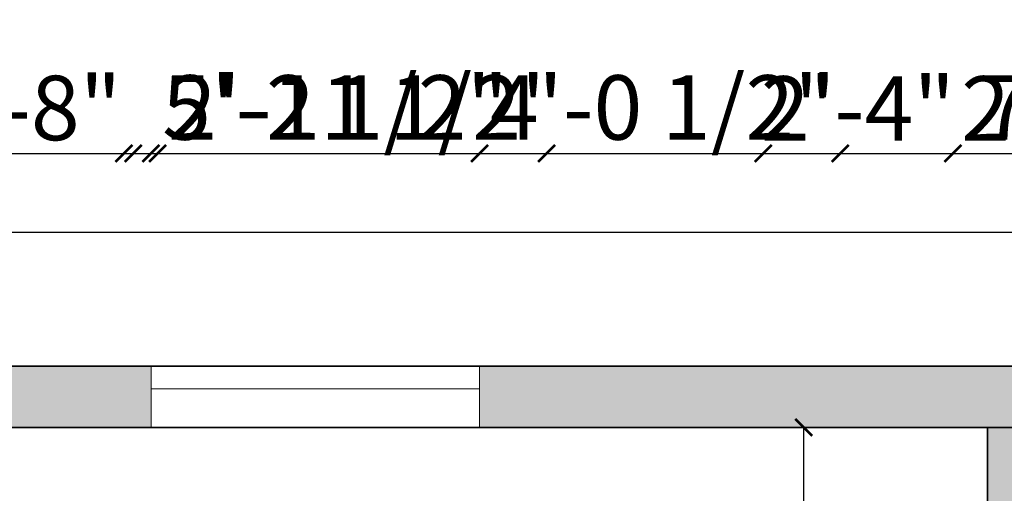
# Model space of a CAD drawing. Units: inches. Extents: x 1704 to 2334, y 1856 to 2559.
# Tile 6 of 10: x 1779 to 1925, y 2489 to 2559. Entities that reach past the tile are written whole.
import ezdxf

# ---------------------------------------------------------------- set-up
doc = ezdxf.new("R2010")
doc.units = ezdxf.units.IN
for name, color, linetype, lineweight in [('A-ANNO-DIMS', 2, 'Continuous', 18), ('A-WALL', 7, 'Continuous', 35), ('WINDOW', 6, 'Continuous', 18)]:
    doc.layers.add(name, color=color, linetype=linetype, lineweight=lineweight)
doc.layers.add('A-WALL-PATT', color=18, linetype='Continuous', lineweight=13, true_color=0x000000)
doc.styles.get("Standard").update_dxf_attribs({"font": 'arial.ttf'})
doc.dimstyles.new('ISO-25', dxfattribs={"dimtxt": 9.5, "dimasz": 2.5, "dimexe": 1.25, "dimexo": 0.625, "dimtad": 1, "dimdec": 0, "dimlunit": 4, "dimtxsty": 'Standard', "dimblk": 'ARCHTICK', "dimcen": 2.5, "dimse1": 1, "dimse2": 1, "dimclrd": 3, "dimadec": 0, "dimazin": 0, "dimtfac": 1, "dimtdec": 0, "dimtmove": 0, "dimatfit": 3, "dimfxl": 1, "dimarcsym": 0})

# ---------------------------------------------------------------- blocks, each defined once
blk = doc.blocks.new('_ArchTick')
at = {"color": 0, "linetype": 'ByBlock', "const_width": 0.15}
blk.add_lwpolyline([(-0.5, -0.5), (0.5, 0.5)], dxfattribs=at)
blk = doc.blocks.new('*D11')
at = {"layer": 'A-ANNO-DIMS', "color": 0, "lineweight": -2, "transparency": 16777216}
blk.add_line((1894.94, 2355.04), (1894.94, 2499.04), dxfattribs=at)
at = {"layer": 'Defpoints', "color": 0, "transparency": 16777216}
for p in [(1894.94, 2499.04), (1905.46, 2499.04), (1905.46, 2355.04)]:
    blk.add_point(p, dxfattribs=at)
at = {"layer": 'A-ANNO-DIMS', "color": 0, "lineweight": -2, "transparency": 16777216, "xscale": 2.5, "yscale": 2.5, "zscale": 2.5}
for p, rotation in [((1894.94, 2499.04), 90), ((1894.94, 2355.04), 270)]:
    blk.add_blockref('_ArchTick', p, dxfattribs=dict(at, rotation=rotation))
at = {"layer": 'A-ANNO-DIMS', "color": 0, "transparency": 16777216, "insert": (1889.55, 2427.04), "char_height": 9.5, "attachment_point": 5, "rotation": 90}
blk.add_mtext("12'", dxfattribs=at)
blk = doc.blocks.new('*D22')
at = {"layer": 'A-ANNO-DIMS', "color": 0, "lineweight": -2, "transparency": 16777216}
blk.add_line((1755.01, 2527.77), (2175.01, 2527.77), dxfattribs=at)
at = {"layer": 'Defpoints', "color": 0, "transparency": 16777216}
for p in [(2175.01, 2527.77), (1755.01, 2508.04), (2175.01, 2508.04)]:
    blk.add_point(p, dxfattribs=at)
at = {"layer": 'A-ANNO-DIMS', "color": 0, "lineweight": -2, "transparency": 16777216, "xscale": 2.5, "yscale": 2.5, "zscale": 2.5, "rotation": 180}
blk.add_blockref('_ArchTick', (1755.01, 2527.77), dxfattribs=at)
at = {"layer": 'A-ANNO-DIMS', "color": 0, "lineweight": -2, "transparency": 16777216, "xscale": 2.5, "yscale": 2.5, "zscale": 2.5}
blk.add_blockref('_ArchTick', (2175.01, 2527.77), dxfattribs=at)
at = {"layer": 'A-ANNO-DIMS', "color": 0, "transparency": 16777216, "insert": (1965.01, 2533.25), "char_height": 9.5, "attachment_point": 5}
blk.add_mtext("35'", dxfattribs=at)
blk = doc.blocks.new('*D43')
at = {"layer": 'A-ANNO-DIMS', "color": 3, "lineweight": -2, "transparency": 16777216}
blk.add_line((1764.01, 2539.39), (1796.13, 2539.39), dxfattribs=at)
at = {"layer": 'Defpoints', "color": 0, "transparency": 16777216}
for p in [(1796.13, 2539.39), (1764.01, 2148.04), (1796.13, 2148.04)]:
    blk.add_point(p, dxfattribs=at)
at = {"layer": 'A-ANNO-DIMS', "color": 3, "lineweight": -2, "transparency": 16777216, "xscale": 2.5, "yscale": 2.5, "zscale": 2.5, "rotation": 180}
blk.add_blockref('_ArchTick', (1764.01, 2539.39), dxfattribs=at)
at = {"layer": 'A-ANNO-DIMS', "color": 3, "lineweight": -2, "transparency": 16777216, "xscale": 2.5, "yscale": 2.5, "zscale": 2.5}
blk.add_blockref('_ArchTick', (1796.13, 2539.39), dxfattribs=at)
at = {"layer": 'A-ANNO-DIMS', "color": 0, "transparency": 16777216, "insert": (1780.07, 2544.86), "char_height": 9.5, "attachment_point": 5}
blk.add_mtext('2\'-8"', dxfattribs=at)
blk = doc.blocks.new('*D48')
at = {"layer": 'A-ANNO-DIMS', "color": 3, "lineweight": -2, "transparency": 16777216}
for p, q in [((1764.01, 2539.39), (1799.73, 2539.39)), ((1799.73, 2539.39), (1858.41, 2539.39))]:
    blk.add_line(p, q, dxfattribs=at)
at = {"layer": 'Defpoints', "color": 0, "transparency": 16777216}
for p in [(1799.73, 2539.39), (1764.01, 2200.93), (1799.73, 2200.93)]:
    blk.add_point(p, dxfattribs=at)
at = {"layer": 'A-ANNO-DIMS', "color": 3, "lineweight": -2, "transparency": 16777216, "xscale": 2.5, "yscale": 2.5, "zscale": 2.5, "rotation": 180}
blk.add_blockref('_ArchTick', (1764.01, 2539.39), dxfattribs=at)
at = {"layer": 'A-ANNO-DIMS', "color": 3, "lineweight": -2, "transparency": 16777216, "xscale": 2.5, "yscale": 2.5, "zscale": 2.5}
blk.add_blockref('_ArchTick', (1799.73, 2539.39), dxfattribs=at)
at = {"layer": 'A-ANNO-DIMS', "color": 0, "transparency": 16777216, "insert": (1830.32, 2544.93), "char_height": 9.5, "attachment_point": 5}
blk.add_mtext('2\'-11 1/2"', dxfattribs=at)
blk = doc.blocks.new('*D53')
at = {"layer": 'A-ANNO-DIMS', "color": 3, "lineweight": -2, "transparency": 16777216}
for p, q in [((1764.01, 1864.5), (1798.75, 1864.5)), ((1798.75, 1864.5), (1857.43, 1864.5))]:
    blk.add_line(p, q, dxfattribs=at)
at = {"layer": 'Defpoints', "color": 0, "transparency": 16777216}
for p in [(1764.01, 2499.04), (1798.75, 2499.04), (1798.75, 1864.5)]:
    blk.add_point(p, dxfattribs=at)
at = {"layer": 'A-ANNO-DIMS', "color": 3, "lineweight": -2, "transparency": 16777216, "xscale": 2.5, "yscale": 2.5, "zscale": 2.5, "rotation": 180}
blk.add_blockref('_ArchTick', (1764.01, 1864.5), dxfattribs=at)
at = {"layer": 'A-ANNO-DIMS', "color": 3, "lineweight": -2, "transparency": 16777216, "xscale": 2.5, "yscale": 2.5, "zscale": 2.5}
blk.add_blockref('_ArchTick', (1798.75, 1864.5), dxfattribs=at)
at = {"layer": 'A-ANNO-DIMS', "color": 0, "transparency": 16777216, "insert": (1829.34, 1870.04), "char_height": 9.5, "attachment_point": 5}
blk.add_mtext('2\'-10 1/2"', dxfattribs=at)
blk = doc.blocks.new('*D54')
at = {"layer": 'A-ANNO-DIMS', "color": 3, "lineweight": -2, "transparency": 16777216}
for p, q in [((1798.75, 2539.39), (1847.17, 2539.39)), ((1847.17, 2539.39), (1898.7, 2539.39))]:
    blk.add_line(p, q, dxfattribs=at)
at = {"layer": 'Defpoints', "color": 0, "transparency": 16777216}
for p in [(1847.17, 2539.39), (1798.75, 2499.04), (1847.17, 2499.04)]:
    blk.add_point(p, dxfattribs=at)
at = {"layer": 'A-ANNO-DIMS', "color": 3, "lineweight": -2, "transparency": 16777216, "xscale": 2.5, "yscale": 2.5, "zscale": 2.5, "rotation": 180}
blk.add_blockref('_ArchTick', (1798.75, 2539.39), dxfattribs=at)
at = {"layer": 'A-ANNO-DIMS', "color": 3, "lineweight": -2, "transparency": 16777216, "xscale": 2.5, "yscale": 2.5, "zscale": 2.5}
blk.add_blockref('_ArchTick', (1847.17, 2539.39), dxfattribs=at)
at = {"layer": 'A-ANNO-DIMS', "color": 0, "transparency": 16777216, "insert": (1874.18, 2544.93), "char_height": 9.5, "attachment_point": 5}
blk.add_mtext('4\'-0 1/2"', dxfattribs=at)
blk = doc.blocks.new('*D62')
at = {"layer": 'A-ANNO-DIMS', "color": 3, "lineweight": -2, "transparency": 16777216}
blk.add_line((1794.77, 2539.39), (1857.04, 2539.39), dxfattribs=at)
at = {"layer": 'Defpoints', "color": 0, "transparency": 16777216}
for p in [(1857.04, 2539.39), (1794.77, 1977.04), (1857.04, 1977.04)]:
    blk.add_point(p, dxfattribs=at)
at = {"layer": 'A-ANNO-DIMS', "color": 3, "lineweight": -2, "transparency": 16777216, "xscale": 2.5, "yscale": 2.5, "zscale": 2.5, "rotation": 180}
blk.add_blockref('_ArchTick', (1794.77, 2539.39), dxfattribs=at)
at = {"layer": 'A-ANNO-DIMS', "color": 3, "lineweight": -2, "transparency": 16777216, "xscale": 2.5, "yscale": 2.5, "zscale": 2.5}
blk.add_blockref('_ArchTick', (1857.04, 2539.39), dxfattribs=at)
at = {"layer": 'A-ANNO-DIMS', "color": 0, "transparency": 16777216, "insert": (1825.9, 2544.93), "char_height": 9.5, "attachment_point": 5}
blk.add_mtext('5\'-2 1/2"', dxfattribs=at)
blk = doc.blocks.new('*D63')
at = {"layer": 'A-ANNO-DIMS', "color": 3, "lineweight": -2, "transparency": 16777216}
blk.add_line((1888.97, 2539.39), (1916.93, 2539.39), dxfattribs=at)
at = {"layer": 'Defpoints', "color": 0, "transparency": 16777216}
for p in [(1916.93, 2539.39), (1888.97, 2153.04), (1916.93, 2153.04)]:
    blk.add_point(p, dxfattribs=at)
at = {"layer": 'A-ANNO-DIMS', "color": 3, "lineweight": -2, "transparency": 16777216, "xscale": 2.5, "yscale": 2.5, "zscale": 2.5, "rotation": 180}
blk.add_blockref('_ArchTick', (1888.97, 2539.39), dxfattribs=at)
at = {"layer": 'A-ANNO-DIMS', "color": 3, "lineweight": -2, "transparency": 16777216, "xscale": 2.5, "yscale": 2.5, "zscale": 2.5}
blk.add_blockref('_ArchTick', (1916.93, 2539.39), dxfattribs=at)
at = {"layer": 'A-ANNO-DIMS', "color": 0, "transparency": 16777216, "insert": (1902.95, 2544.78), "char_height": 9.5, "attachment_point": 5}
blk.add_mtext('2\'-4"', dxfattribs=at)
blk = doc.blocks.new('*D74')
at = {"layer": 'A-ANNO-DIMS', "color": 3, "lineweight": -2, "transparency": 16777216}
blk.add_line((1916.93, 2539.39), (1948.02, 2539.39), dxfattribs=at)
at = {"layer": 'Defpoints', "color": 0, "transparency": 16777216}
for p in [(1948.02, 2539.39), (1916.93, 2153.04), (1948.02, 2153.04)]:
    blk.add_point(p, dxfattribs=at)
at = {"layer": 'A-ANNO-DIMS', "color": 3, "lineweight": -2, "transparency": 16777216, "xscale": 2.5, "yscale": 2.5, "zscale": 2.5, "rotation": 180}
blk.add_blockref('_ArchTick', (1916.93, 2539.39), dxfattribs=at)
at = {"layer": 'A-ANNO-DIMS', "color": 3, "lineweight": -2, "transparency": 16777216, "xscale": 2.5, "yscale": 2.5, "zscale": 2.5}
blk.add_blockref('_ArchTick', (1948.02, 2539.39), dxfattribs=at)
at = {"layer": 'A-ANNO-DIMS', "color": 0, "transparency": 16777216, "insert": (1932.47, 2544.78), "char_height": 9.5, "attachment_point": 5}
blk.add_mtext('2\'-7"', dxfattribs=at)
blk = doc.blocks.new('*D80')
at = {"layer": 'A-ANNO-DIMS', "color": 3, "lineweight": -2, "transparency": 16777216}
blk.add_line((1900.32, 2539.39), (1993.01, 2539.39), dxfattribs=at)
at = {"layer": 'Defpoints', "color": 0, "transparency": 16777216}
for p in [(1993.01, 2539.39), (1900.32, 2273.04), (1993.01, 2273.04)]:
    blk.add_point(p, dxfattribs=at)
at = {"layer": 'A-ANNO-DIMS', "color": 3, "lineweight": -2, "transparency": 16777216, "xscale": 2.5, "yscale": 2.5, "zscale": 2.5, "rotation": 180}
blk.add_blockref('_ArchTick', (1900.32, 2539.39), dxfattribs=at)
at = {"layer": 'A-ANNO-DIMS', "color": 3, "lineweight": -2, "transparency": 16777216, "xscale": 2.5, "yscale": 2.5, "zscale": 2.5}
blk.add_blockref('_ArchTick', (1993.01, 2539.39), dxfattribs=at)
at = {"layer": 'A-ANNO-DIMS', "color": 0, "transparency": 16777216, "insert": (1946.66, 2544.93), "char_height": 9.5, "attachment_point": 5}
blk.add_mtext('7\'-8 1/2"', dxfattribs=at)

msp = doc.modelspace()

# ---------------------------------------------------------------- hatches: boundary and pattern name
at = {"layer": 'A-WALL-PATT'}
h = msp.add_hatch(color=256, dxfattribs=at)
h.dxf.hatch_style = 1
h.paths.add_polyline_path([(1764.01, 2204.96), (1755.01, 2204.96), (1755.01, 2115.31), (1764.01, 2115.31)])
h.paths.add_polyline_path([(1764.01, 2076.84), (1755.01, 2076.84), (1755.01, 1968.04), (1794.77, 1968.04), (1794.77, 1977.04), (1764.01, 1977.04)])
h.paths.add_polyline_path([(1927.01, 1977.04), (1927.01, 2069.24), (1993.01, 2069.24), (1993.01, 1977.04)], flags=16)
h.paths.add_polyline_path([(1927.01, 2074.24), (1927.01, 2148.04), (1993.01, 2148.04), (1993.01, 2074.24)], flags=16)
h.paths.add_polyline_path([(1764.01, 2318.65), (1755.01, 2318.65), (1755.01, 2247.44), (1764.01, 2247.44)])
h.paths.add_polyline_path([(1764.01, 2499.04), (1798.75, 2499.04), (1798.75, 2508.04), (1755.01, 2508.04), (1755.01, 2336.43), (1764.01, 2336.43)])
h.paths.add_polyline_path([(1950.56, 2508.04), (1847.17, 2508.04), (1847.17, 2499.04), (1950.56, 2499.04)])
h.paths.add_polyline_path([(2059.64, 2508.04), (1975.68, 2508.04), (1975.68, 2499.04), (2059.64, 2499.04)])
h.paths.add_polyline_path([(2175.01, 2508.04), (2108.25, 2508.04), (2108.25, 2499.04), (2166.01, 2499.04), (2166.01, 1977.04), (2166.01, 1972.26), (2166.01, 1968.04), (2175.01, 1968.04)])
h.paths.add_polyline_path([(2166.01, 2319.04), (1993.01, 2319.04), (1993.01, 2273.04), (1998.01, 2273.04), (1998.01, 2314.04), (2166.01, 2314.04)])
h.paths.add_polyline_path([(2054.53, 2117.04), (1998.01, 2117.04), (1998.01, 2112.04), (2054.53, 2112.04)])
h.paths.add_polyline_path([(2166.01, 2117.04), (2105.53, 2117.04), (2105.53, 2112.04), (2166.01, 2112.04)])
h.paths.add_polyline_path([(1927.01, 2499.04), (1922.01, 2499.04), (1922.01, 2355.04), (1764.01, 2355.04), (1764.01, 2350.04), (1804.01, 2350.04), (1804.01, 2278.04), (1764.01, 2278.04), (1764.01, 2273.04), (1870.51, 2273.04), (1870.51, 2278.04), (1870.51, 2350.04), (1865.51, 2350.04), (1865.51, 2278.04), (1809.01, 2278.04), (1809.01, 2350.04), (1922.01, 2350.04), (1927.01, 2350.04), (1998.01, 2350.04), (1998.01, 2499.04), (1993.01, 2499.04), (1993.01, 2355.04), (1927.01, 2355.04)])
h.paths.add_polyline_path([(2131.1, 2203.36), (2144.85, 2203.36), (2144.85, 2212.38), (2131.1, 2212.38)], flags=25)
h.paths.add_polyline_path([(2010.94, 2265.21), (2036.85, 2265.21), (2036.85, 2274.23), (2010.94, 2274.23)], flags=9)
h.paths.add_polyline_path([(2010.9, 2274.71), (2056.95, 2274.71), (2056.95, 2284.04), (2010.9, 2284.04)], flags=25)
h.paths.add_polyline_path([(2003.27, 2440.18), (2049.79, 2440.18), (2049.79, 2449.51), (2003.27, 2449.51)], flags=9)
h.paths.add_polyline_path([(1934.96, 2428.22), (1967.48, 2428.22), (1967.48, 2437.55), (1934.96, 2437.55)], flags=25)
h.paths.add_polyline_path([(1778.93, 2466.23), (1827.79, 2466.23), (1827.79, 2475.56), (1778.93, 2475.56)], flags=25)
h.paths.add_polyline_path([(1938.32, 2043.05), (1970.37, 2043.05), (1970.37, 2052.39), (1938.32, 2052.39)], flags=8)
h.paths.add_polyline_path([(1932.21, 2095.38), (1956.75, 2095.38), (1956.75, 2104.56), (1932.21, 2104.56)], flags=8)
h.paths.add_polyline_path([(1888.97, 2148.04), (1888.97, 2153.04), (1764.01, 2153.04), (1764.01, 2148.04)])
h.paths.add_polyline_path([(1922.01, 2059.61), (1927.01, 2059.61), (1927.01, 2044.47), (1922.01, 2044.47), (1922.01, 1977.04), (1857.04, 1977.04), (1857.04, 1968.04), (1998.01, 1968.04), (1998.01, 1977.04), (1998.01, 2153.04), (1916.93, 2153.04), (1916.93, 2148.04), (1922.01, 2148.04)])

# ---------------------------------------------------------------- linework, layer by layer
at = {"layer": 'A-WALL'}
for p, q in [((1764.01, 2499.04), (2166.01, 2499.04)), ((1922.01, 2419.48), (1922.01, 2499.04))]:
    msp.add_line(p, q, dxfattribs=at)
msp.add_lwpolyline([(1998.01, 1968.04), (1755.01, 1968.04), (1755.01, 2508.04), (2175.01, 2508.04), (2175.01, 1968.04), (2166.01, 1968.04)], dxfattribs=at)
at = {"layer": 'WINDOW'}
for p, q in [((1798.75, 2508.04), (1798.75, 2499.04)), ((1847.17, 2508.04), (1798.75, 2508.04)), ((1847.17, 2499.04), (1847.17, 2508.04)), ((1847.17, 2504.74), (1798.75, 2504.74)), ((1798.75, 2499.04), (1847.17, 2499.04)), ((1847.17, 2499.04), (1798.75, 2499.04)), ((1847.17, 2499.04), (1798.75, 2499.04))]:
    msp.add_line(p, q, dxfattribs=at)

# ---------------------------------------------------------------- dimensions: what is measured, and where the dimension line sits
at = {"layer": 'A-ANNO-DIMS'}
for base, p1, p2, override, picture, middle in [((1799.73, 2539.39), (1764.01, 2200.93), (1799.73, 2200.93), {"dimdec": 1, "dimlfac": 1, "dimrnd": 0, "dimzin": 1, "dimdsep": 46, "dimlunit": 4, "dimfrac": 2}, '*D48', (1830.32, 2544.93)), ((1857.04, 2539.39), (1794.77, 1977.04), (1857.04, 1977.04), {"dimdec": 1, "dimlfac": 1, "dimrnd": 0, "dimzin": 1, "dimdsep": 46, "dimlunit": 4, "dimfrac": 2}, '*D62', (1825.9, 2544.93)), ((1847.17, 2539.39), (1798.75, 2499.04), (1847.17, 2499.04), {"dimdec": 1, "dimlfac": 1, "dimrnd": 0, "dimzin": 1, "dimdsep": 46, "dimlunit": 4, "dimfrac": 2}, '*D54', (1874.18, 2544.93)), ((1993.01, 2539.39), (1900.32, 2273.04), (1993.01, 2273.04), {"dimdec": 1, "dimlfac": 1, "dimrnd": 0, "dimzin": 1, "dimdsep": 46, "dimlunit": 4, "dimfrac": 2}, '*D80', (1946.66, 2544.93)), ((1796.13, 2539.39), (1764.01, 2148.04), (1796.13, 2148.04), {"dimdec": 1, "dimlfac": 1, "dimrnd": 0, "dimzin": 1, "dimdsep": 46, "dimlunit": 4, "dimfrac": 2}, '*D43', (1780.07, 2544.86)), ((1916.93, 2539.39), (1888.97, 2153.04), (1916.93, 2153.04), {"dimdec": 1, "dimlfac": 1, "dimrnd": 0, "dimzin": 1, "dimdsep": 46, "dimlunit": 4, "dimfrac": 2}, '*D63', (1902.95, 2544.78)), ((1948.02, 2539.39), (1916.93, 2153.04), (1948.02, 2153.04), {"dimdec": 1, "dimlfac": 1, "dimrnd": 0, "dimzin": 1, "dimdsep": 46, "dimlunit": 4, "dimfrac": 2}, '*D74', (1932.47, 2544.78)), ((2175.01, 2527.77), (1755.01, 2508.04), (2175.01, 2508.04), {"dimclrd": 0, "dimclre": 0, "dimclrt": 0}, '*D22', (1965.01, 2533.25)), ((1798.75, 1864.5), (1764.01, 2499.04), (1798.75, 2499.04), {"dimdec": 1, "dimlfac": 1, "dimrnd": 0, "dimzin": 1, "dimdsep": 46, "dimlunit": 4, "dimfrac": 2}, '*D53', (1829.34, 1870.04))]:
    dim = msp.add_linear_dim(base=base, p1=p1, p2=p2, dimstyle='ISO-25', override=override, dxfattribs=at)
    dim.commit()
    dim.dimension.update_dxf_attribs({"geometry": picture, "text_midpoint": middle})
dim = msp.add_linear_dim(base=(1894.94, 2499.04), p1=(1905.46, 2355.04), p2=(1905.46, 2499.04), angle=90, dimstyle='ISO-25', override={"dimclrd": 0, "dimclre": 0, "dimclrt": 0}, dxfattribs=at)
dim.commit()
dim.dimension.update_dxf_attribs({"geometry": '*D11', "text_midpoint": (1889.55, 2427.04)})

doc.saveas('drawing.dxf')
